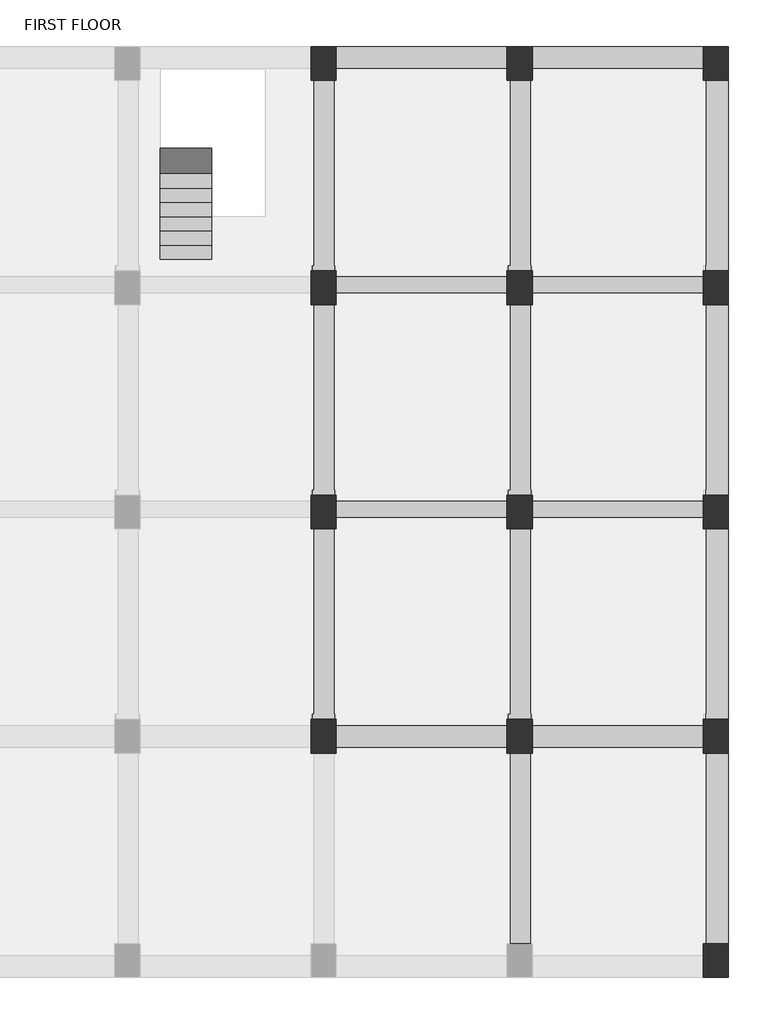
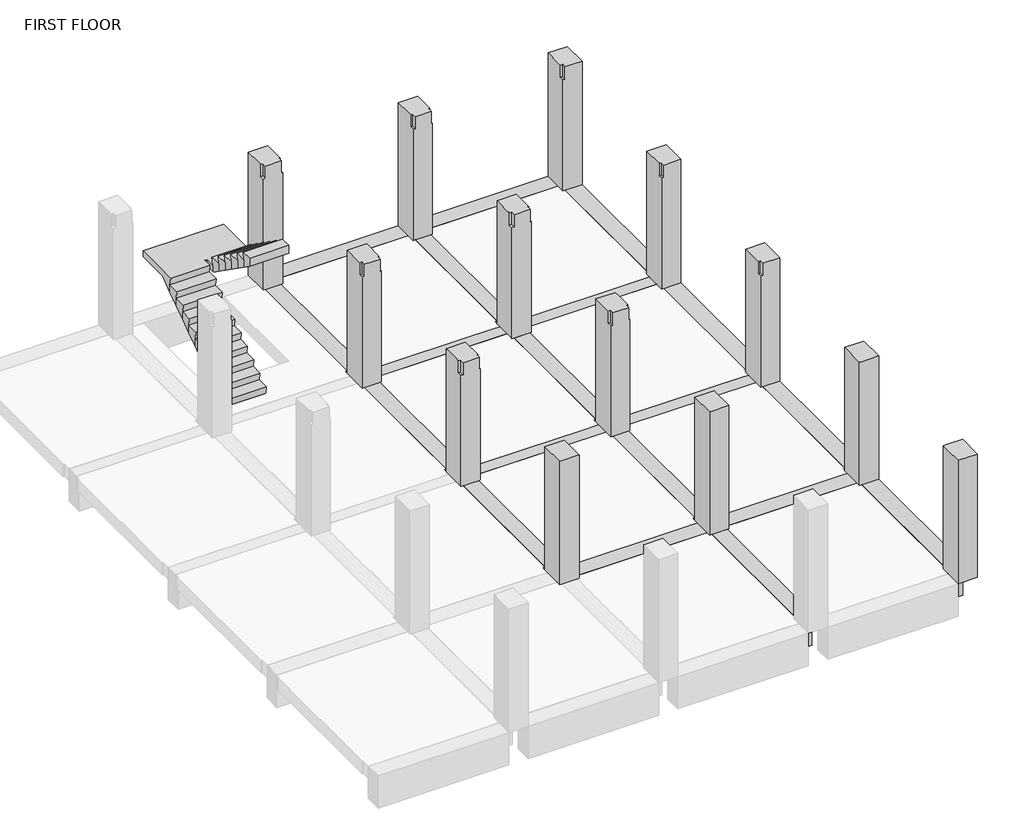
# One storey, part 4 of 4: 19 beams, 13 columns, 1 stair flight.
"""IFC4 building model written with IfcOpenShell, lengths in millimetres."""

from ifc_helpers import new_model, si_unit, origin, place, context, project, spatial, faceted_brep, element, save

model = new_model("IFC4")

# Units and contexts
model_context = context("Model", 3, world=origin())
ifc_project = project(units=[si_unit("LENGTHUNIT", "METRE", prefix="MILLI")], contexts=[model_context])

# Site, building, storey
site = spatial("IfcSite", under=ifc_project)
building = spatial("IfcBuilding", under=site)
storey = spatial("IfcBuildingStorey", under=building, Name="FIRST FLOOR", Elevation=3048.0)

# Beams
placement = place(None, origin())
element("IfcBeam", 1, ObjectType="M_Concrete-Rectangular Beam : 400 x 800mm", at=placement, inside=storey, context=model_context, shape_type="Brep", body=[
    faceted_brep([(7955.1115906, 15703.1212443, 3048.0), (8355.1115906, 15703.1212443, 3048.0), (8355.1115906, 19103.1212443, 3048.0), (7955.1115906, 19103.1212443, 3048.0), (7955.1115906, 15803.1212443, 3048.0), (7955.1115906, 15703.1212443, 2248.0), (7955.1115906, 19103.1212443, 2248.0), (8355.1115906, 15703.1212443, 2248.0), (8355.1115906, 19103.1212443, 2248.0)], [[[0, 1, 2, 3, 4]], [[5, 0, 4, 3, 6]], [[7, 5, 6, 8]], [[1, 7, 8, 2]], [[2, 8, 6, 3]], [[1, 0, 5, 7]]]),
])
element("IfcBeam", 2, ObjectType="M_Concrete-Rectangular Beam : 400 x 800mm", at=placement, inside=storey, context=model_context, shape_type="Brep", body=[
    faceted_brep([(7955.1115906, 11703.1212443, 3048.0), (8355.1115906, 11703.1212443, 3048.0), (8355.1115906, 15103.1212443, 3048.0), (7955.1115906, 15103.1212443, 3048.0), (7955.1115906, 11803.1212443, 3048.0), (7955.1115906, 11703.1212443, 2248.0), (7955.1115906, 15103.1212443, 2248.0), (8355.1115906, 11703.1212443, 2248.0), (8355.1115906, 15103.1212443, 2248.0)], [[[0, 1, 2, 3, 4]], [[5, 0, 4, 3, 6]], [[7, 5, 6, 8]], [[1, 7, 8, 2]], [[2, 8, 6, 3]], [[1, 0, 5, 7]]]),
])
element("IfcBeam", 3, ObjectType="M_Concrete-Rectangular Beam : 400 x 800mm", at=placement, inside=storey, context=model_context, shape_type="Brep", body=[
    faceted_brep([(7955.1115906, 7703.1212443, 3048.0), (8355.1115906, 7703.1212443, 3048.0), (8355.1115906, 11103.1212443, 3048.0), (7955.1115906, 11103.1212443, 3048.0), (7955.1115906, 7803.1212443, 3048.0), (7955.1115906, 7703.1212443, 2248.0), (7955.1115906, 11103.1212443, 2248.0), (8355.1115906, 7703.1212443, 2248.0), (8355.1115906, 11103.1212443, 2248.0)], [[[0, 1, 2, 3, 4]], [[5, 0, 4, 3, 6]], [[7, 5, 6, 8]], [[1, 7, 8, 2]], [[1, 0, 5, 7]], [[3, 2, 8, 6]]]),
])
element("IfcBeam", 4, ObjectType="M_Concrete-Rectangular Beam : 400 x 800mm", at=placement, inside=storey, context=model_context, shape_type="Brep", body=[
    faceted_brep([(8355.1115906, 7103.1212443, 3048.0), (7955.1115906, 7103.1212443, 3048.0), (7955.1115906, 3703.1212443, 3048.0), (8355.1115906, 3703.1212443, 3048.0), (7955.1115906, 7103.1212443, 2748.0), (7955.1115906, 7103.1212443, 2248.0), (7955.1115906, 3703.1212443, 2248.0), (7955.1115906, 3703.1212443, 2748.0), (8355.1115906, 7103.1212443, 2248.0), (8355.1115906, 3703.1212443, 2248.0)], [[[0, 1, 2, 3]], [[1, 4, 5, 6, 7, 2]], [[5, 8, 9, 6]], [[8, 0, 3, 9]], [[0, 8, 5, 4, 1]], [[3, 2, 7, 6, 9]]]),
])
element("IfcBeam", 5, ObjectType="M_Concrete-Rectangular Beam : 400 x 800mm", at=placement, inside=storey, context=model_context, shape_type="Brep", body=[
    faceted_brep([(1355.1115906, 19703.1212443, 3048.0), (1355.1115906, 19303.1212443, 3048.0), (4405.1115906, 19303.1212443, 3048.0), (4405.1115906, 19703.1212443, 3048.0), (1355.1115906, 19303.1212443, 2748.0), (1355.1115906, 19303.1212443, 2248.0), (4405.1115906, 19303.1212443, 2248.0), (4405.1115906, 19303.1212443, 2748.0), (1355.1115906, 19703.1212443, 2248.0), (4405.1115906, 19703.1212443, 2248.0)], [[[0, 1, 2, 3]], [[1, 4, 5, 6, 7, 2]], [[5, 8, 9, 6]], [[8, 0, 3, 9]], [[1, 0, 8, 5, 4]], [[3, 2, 7, 6, 9]]]),
])
element("IfcBeam", 6, ObjectType="M_Concrete-Rectangular Beam : 400 x 800mm", at=placement, inside=storey, context=model_context, shape_type="Brep", body=[
    faceted_brep([(4855.1115906, 19703.1212443, 3048.0), (4855.1115906, 19303.1212443, 3048.0), (7905.1115906, 19303.1212443, 3048.0), (7905.1115906, 19703.1212443, 3048.0), (4855.1115906, 19303.1212443, 2748.0), (4855.1115906, 19303.1212443, 2248.0), (7905.1115906, 19303.1212443, 2248.0), (7905.1115906, 19303.1212443, 2748.0), (4855.1115906, 19703.1212443, 2248.0), (7905.1115906, 19703.1212443, 2248.0)], [[[0, 1, 2, 3]], [[1, 4, 5, 6, 7, 2]], [[5, 8, 9, 6]], [[8, 0, 3, 9]], [[1, 0, 8, 5, 4]], [[3, 2, 7, 6, 9]]]),
])
element("IfcBeam", 7, ObjectType="M_Concrete-Rectangular Beam : 400 x 800mm", at=placement, inside=storey, context=model_context, shape_type="Brep", body=[
    faceted_brep([(1330.1115906, 15703.1212443, 3048.0), (1330.1115906, 15803.1212443, 3048.0), (1330.1115906, 19103.1212443, 3048.0), (955.1115906, 19103.1212443, 3048.0), (955.1115906, 15803.1212443, 3048.0), (930.1115906, 15803.1212443, 3048.0), (930.1115906, 15703.1212443, 3048.0), (930.1115906, 19103.1212443, 2248.0), (930.1115906, 15703.1212443, 2248.0), (930.1115906, 15803.1212443, 2748.0), (930.1115906, 19103.1212443, 2748.0), (1330.1115906, 19103.1212443, 2248.0), (1330.1115906, 15703.1212443, 2248.0), (955.1115906, 19103.1212443, 2748.0), (955.1115906, 15803.1212443, 2748.0)], [[[0, 1, 2, 3, 4, 5, 6]], [[7, 8, 6, 5, 9, 10]], [[7, 11, 12, 8]], [[11, 2, 1, 0, 12]], [[2, 11, 7, 10, 13, 3]], [[0, 6, 8, 12]], [[9, 14, 13, 10]], [[14, 4, 3, 13]], [[4, 14, 9, 5]]]),
])
element("IfcBeam", 8, ObjectType="M_Concrete-Rectangular Beam : 400 x 800mm", at=placement, inside=storey, context=model_context, shape_type="Brep", body=[
    faceted_brep([(1330.1115906, 11703.1212443, 3048.0), (1330.1115906, 11803.1212443, 3048.0), (1330.1115906, 15103.1212443, 3048.0), (955.1115906, 15103.1212443, 3048.0), (955.1115906, 11803.1212443, 3048.0), (930.1115906, 11803.1212443, 3048.0), (930.1115906, 11703.1212443, 3048.0), (930.1115906, 15103.1212443, 2248.0), (930.1115906, 11703.1212443, 2248.0), (930.1115906, 11803.1212443, 2748.0), (930.1115906, 15103.1212443, 2748.0), (1330.1115906, 15103.1212443, 2248.0), (1330.1115906, 11703.1212443, 2248.0), (955.1115906, 15103.1212443, 2748.0), (955.1115906, 11803.1212443, 2748.0)], [[[0, 1, 2, 3, 4, 5, 6]], [[7, 8, 6, 5, 9, 10]], [[8, 7, 11, 12]], [[2, 1, 0, 12, 11]], [[2, 11, 7, 10, 13, 3]], [[0, 6, 8, 12]], [[9, 14, 13, 10]], [[14, 4, 3, 13]], [[4, 14, 9, 5]]]),
])
element("IfcBeam", 9, ObjectType="M_Concrete-Rectangular Beam : 400 x 800mm", at=placement, inside=storey, context=model_context, shape_type="Brep", body=[
    faceted_brep([(1330.1115906, 7703.1212443, 3048.0), (1330.1115906, 7803.1212443, 3048.0), (1330.1115906, 11103.1212443, 3048.0), (955.1115906, 11103.1212443, 3048.0), (955.1115906, 7803.1212443, 3048.0), (930.1115906, 7803.1212443, 3048.0), (930.1115906, 7703.1212443, 3048.0), (930.1115906, 11103.1212443, 2248.0), (930.1115906, 7703.1212443, 2248.0), (930.1115906, 7803.1212443, 2748.0), (930.1115906, 11103.1212443, 2748.0), (1330.1115906, 11103.1212443, 2248.0), (1330.1115906, 7703.1212443, 2248.0), (955.1115906, 11103.1212443, 2748.0), (955.1115906, 7803.1212443, 2748.0)], [[[0, 1, 2, 3, 4, 5, 6]], [[7, 8, 6, 5, 9, 10]], [[7, 11, 12, 8]], [[11, 2, 1, 0, 12]], [[2, 11, 7, 10, 13, 3]], [[0, 6, 8, 12]], [[9, 14, 13, 10]], [[14, 4, 3, 13]], [[4, 14, 9, 5]]]),
])
element("IfcBeam", 10, ObjectType="M_Concrete-Rectangular Beam : 400 x 800mm", at=placement, inside=storey, context=model_context, shape_type="Brep", body=[
    faceted_brep([(4830.1115906, 15703.1212443, 3048.0), (4830.1115906, 15803.1212443, 3048.0), (4830.1115906, 19103.1212443, 3048.0), (4455.1115906, 19103.1212443, 3048.0), (4455.1115906, 15803.1212443, 3048.0), (4430.1115906, 15803.1212443, 3048.0), (4430.1115906, 15703.1212443, 3048.0), (4430.1115906, 19103.1212443, 2248.0), (4430.1115906, 15703.1212443, 2248.0), (4430.1115906, 15803.1212443, 2748.0), (4430.1115906, 19103.1212443, 2748.0), (4830.1115906, 19103.1212443, 2248.0), (4830.1115906, 15703.1212443, 2248.0), (4455.1115906, 19103.1212443, 2748.0), (4455.1115906, 15803.1212443, 2748.0)], [[[0, 1, 2, 3, 4, 5, 6]], [[7, 8, 6, 5, 9, 10]], [[8, 7, 11, 12]], [[2, 1, 0, 12, 11]], [[2, 11, 7, 10, 13, 3]], [[0, 6, 8, 12]], [[9, 14, 13, 10]], [[14, 4, 3, 13]], [[4, 14, 9, 5]]]),
])
element("IfcBeam", 11, ObjectType="M_Concrete-Rectangular Beam : 400 x 800mm", at=placement, inside=storey, context=model_context, shape_type="Brep", body=[
    faceted_brep([(4830.1115906, 11703.1212443, 3048.0), (4830.1115906, 11803.1212443, 3048.0), (4830.1115906, 15103.1212443, 3048.0), (4455.1115906, 15103.1212443, 3048.0), (4455.1115906, 11803.1212443, 3048.0), (4430.1115906, 11803.1212443, 3048.0), (4430.1115906, 11703.1212443, 3048.0), (4430.1115906, 15103.1212443, 2248.0), (4430.1115906, 11703.1212443, 2248.0), (4430.1115906, 11803.1212443, 2748.0), (4430.1115906, 15103.1212443, 2748.0), (4830.1115906, 15103.1212443, 2248.0), (4830.1115906, 11703.1212443, 2248.0), (4455.1115906, 15103.1212443, 2748.0), (4455.1115906, 11803.1212443, 2748.0)], [[[0, 1, 2, 3, 4, 5, 6]], [[7, 8, 6, 5, 9, 10]], [[7, 11, 12, 8]], [[11, 2, 1, 0, 12]], [[2, 11, 7, 10, 13, 3]], [[0, 6, 8, 12]], [[9, 14, 13, 10]], [[14, 4, 3, 13]], [[4, 14, 9, 5]]]),
])
element("IfcBeam", 12, ObjectType="M_Concrete-Rectangular Beam : 400 x 800mm", at=placement, inside=storey, context=model_context, shape_type="Brep", body=[
    faceted_brep([(4430.1115906, 7703.1212443, 3048.0), (4830.1115906, 7703.1212443, 3048.0), (4830.1115906, 7803.1212443, 3048.0), (4830.1115906, 11103.1212443, 3048.0), (4455.1115906, 11103.1212443, 3048.0), (4455.1115906, 7803.1212443, 3048.0), (4430.1115906, 7803.1212443, 3048.0), (4430.1115906, 7703.1212443, 2248.0), (4430.1115906, 7803.1212443, 2748.0), (4430.1115906, 11103.1212443, 2748.0), (4430.1115906, 11103.1212443, 2248.0), (4830.1115906, 7703.1212443, 2248.0), (4830.1115906, 11103.1212443, 2248.0), (4455.1115906, 11103.1212443, 2748.0), (4455.1115906, 7803.1212443, 2748.0)], [[[0, 1, 2, 3, 4, 5, 6]], [[7, 0, 6, 8, 9, 10]], [[11, 7, 10, 12]], [[1, 11, 12, 3, 2]], [[1, 0, 7, 11]], [[12, 10, 9, 13, 4, 3]], [[8, 14, 13, 9]], [[14, 5, 4, 13]], [[5, 14, 8, 6]]]),
])
element("IfcBeam", 13, ObjectType="M_Concrete-Rectangular Beam : 400 x 800mm", at=placement, inside=storey, context=model_context, shape_type="Brep", body=[
    faceted_brep([(4830.1115906, 3703.1212443, 3048.0), (4830.1115906, 7103.1212443, 3048.0), (4455.1115906, 7103.1212443, 3048.0), (4455.1115906, 3703.1212443, 3048.0), (4430.1115906, 7103.1212443, 2248.0), (4430.1115906, 3703.1212443, 2248.0), (4430.1115906, 3703.1212443, 2748.0), (4430.1115906, 7103.1212443, 2748.0), (4830.1115906, 7103.1212443, 2248.0), (4830.1115906, 3703.1212443, 2248.0), (4830.1115906, 7103.1212443, 2748.0), (4830.1115906, 3703.1212443, 2748.0), (4455.1115906, 7103.1212443, 2748.0), (4455.1115906, 3703.1212443, 2748.0)], [[[0, 1, 2, 3]], [[4, 5, 6, 7]], [[4, 8, 9, 5]], [[8, 10, 1, 0, 11, 9]], [[1, 10, 8, 4, 7, 12, 2]], [[5, 9, 11, 0, 3, 13, 6]], [[13, 12, 7, 6]], [[12, 13, 3, 2]]]),
])
element("IfcBeam", 14, ObjectType="M_Concrete-Rectangular Beam : 400 x 800mm", at=placement, inside=storey, context=model_context, shape_type="Brep", body=[
    faceted_brep([(4405.1115906, 15603.1212443, 3048.0), (1355.1115906, 15603.1212443, 3048.0), (1355.1115906, 15303.1212443, 3048.0), (4405.1115906, 15303.1212443, 3048.0), (1355.1115906, 15203.1212443, 2248.0), (4405.1115906, 15203.1212443, 2248.0), (4405.1115906, 15203.1212443, 2748.0), (1355.1115906, 15203.1212443, 2748.0), (1355.1115906, 15603.1212443, 2248.0), (4405.1115906, 15603.1212443, 2248.0), (1355.1115906, 15603.1212443, 2748.0), (4405.1115906, 15603.1212443, 2748.0), (1355.1115906, 15303.1212443, 2748.0), (4405.1115906, 15303.1212443, 2748.0)], [[[0, 1, 2, 3]], [[4, 5, 6, 7]], [[4, 8, 9, 5]], [[8, 10, 1, 0, 11, 9]], [[8, 4, 7, 12, 2, 1, 10]], [[5, 9, 11, 0, 3, 13, 6]], [[13, 12, 7, 6]], [[12, 13, 3, 2]]]),
])
element("IfcBeam", 15, ObjectType="M_Concrete-Rectangular Beam : 400 x 800mm", at=placement, inside=storey, context=model_context, shape_type="Brep", body=[
    faceted_brep([(7905.1115906, 15603.1212443, 3048.0), (4855.1115906, 15603.1212443, 3048.0), (4855.1115906, 15303.1212443, 3048.0), (7905.1115906, 15303.1212443, 3048.0), (4855.1115906, 15203.1212443, 2248.0), (7905.1115906, 15203.1212443, 2248.0), (7905.1115906, 15203.1212443, 2748.0), (4855.1115906, 15203.1212443, 2748.0), (4855.1115906, 15603.1212443, 2248.0), (7905.1115906, 15603.1212443, 2248.0), (4855.1115906, 15603.1212443, 2748.0), (7905.1115906, 15603.1212443, 2748.0), (4855.1115906, 15303.1212443, 2748.0), (7905.1115906, 15303.1212443, 2748.0)], [[[0, 1, 2, 3]], [[4, 5, 6, 7]], [[4, 8, 9, 5]], [[8, 10, 1, 0, 11, 9]], [[8, 4, 7, 12, 2, 1, 10]], [[5, 9, 11, 0, 3, 13, 6]], [[13, 12, 7, 6]], [[12, 13, 3, 2]]]),
])
element("IfcBeam", 16, ObjectType="M_Concrete-Rectangular Beam : 400 x 800mm", at=placement, inside=storey, context=model_context, shape_type="Brep", body=[
    faceted_brep([(7905.1115906, 11603.1212443, 3048.0), (4855.1115906, 11603.1212443, 3048.0), (4855.1115906, 11303.1212443, 3048.0), (7905.1115906, 11303.1212443, 3048.0), (4855.1115906, 11603.1212443, 2248.0), (4855.1115906, 11603.1212443, 2748.0), (7905.1115906, 11603.1212443, 2748.0), (7905.1115906, 11603.1212443, 2248.0), (4855.1115906, 11203.1212443, 2248.0), (7905.1115906, 11203.1212443, 2248.0), (7905.1115906, 11203.1212443, 2748.0), (4855.1115906, 11203.1212443, 2748.0), (4855.1115906, 11303.1212443, 2748.0), (7905.1115906, 11303.1212443, 2748.0)], [[[0, 1, 2, 3]], [[4, 5, 1, 0, 6, 7]], [[8, 4, 7, 9]], [[8, 9, 10, 11]], [[1, 5, 4, 8, 11, 12, 2]], [[7, 6, 0, 3, 13, 10, 9]], [[13, 12, 11, 10]], [[12, 13, 3, 2]]]),
])
element("IfcBeam", 17, ObjectType="M_Concrete-Rectangular Beam : 400 x 800mm", at=placement, inside=storey, context=model_context, shape_type="Brep", body=[
    faceted_brep([(4405.1115906, 11603.1212443, 3048.0), (1355.1115906, 11603.1212443, 3048.0), (1355.1115906, 11303.1212443, 3048.0), (4405.1115906, 11303.1212443, 3048.0), (1355.1115906, 11603.1212443, 2248.0), (1355.1115906, 11603.1212443, 2748.0), (4405.1115906, 11603.1212443, 2748.0), (4405.1115906, 11603.1212443, 2248.0), (1355.1115906, 11203.1212443, 2248.0), (4405.1115906, 11203.1212443, 2248.0), (4405.1115906, 11203.1212443, 2748.0), (1355.1115906, 11203.1212443, 2748.0), (1355.1115906, 11303.1212443, 2748.0), (4405.1115906, 11303.1212443, 2748.0)], [[[0, 1, 2, 3]], [[4, 5, 1, 0, 6, 7]], [[8, 4, 7, 9]], [[8, 9, 10, 11]], [[1, 5, 4, 8, 11, 12, 2]], [[7, 6, 0, 3, 13, 10, 9]], [[13, 12, 11, 10]], [[12, 13, 3, 2]]]),
])
element("IfcBeam", 18, ObjectType="M_Concrete-Rectangular Beam : 400 x 800mm", at=placement, inside=storey, context=model_context, shape_type="Brep", body=[
    faceted_brep([(1355.1115906, 7603.1212443, 3048.0), (1355.1115906, 7203.1212443, 3048.0), (4405.1115906, 7203.1212443, 3048.0), (4405.1115906, 7603.1212443, 3048.0), (1355.1115906, 7203.1212443, 2748.0), (1355.1115906, 7203.1212443, 2248.0), (4405.1115906, 7203.1212443, 2248.0), (4405.1115906, 7203.1212443, 2748.0), (1355.1115906, 7603.1212443, 2248.0), (4405.1115906, 7603.1212443, 2248.0), (1355.1115906, 7603.1212443, 2748.0), (4405.1115906, 7603.1212443, 2748.0)], [[[0, 1, 2, 3]], [[1, 4, 5, 6, 7, 2]], [[5, 8, 9, 6]], [[8, 10, 0, 3, 11, 9]], [[1, 0, 10, 8, 5, 4]], [[3, 2, 7, 6, 9, 11]]]),
])
element("IfcBeam", 19, ObjectType="M_Concrete-Rectangular Beam : 400 x 800mm", at=placement, inside=storey, context=model_context, shape_type="Brep", body=[
    faceted_brep([(4855.1115906, 7603.1212443, 3048.0), (4855.1115906, 7203.1212443, 3048.0), (7905.1115906, 7203.1212443, 3048.0), (7905.1115906, 7603.1212443, 3048.0), (4855.1115906, 7203.1212443, 2748.0), (4855.1115906, 7203.1212443, 2248.0), (7905.1115906, 7203.1212443, 2248.0), (7905.1115906, 7203.1212443, 2748.0), (4855.1115906, 7603.1212443, 2248.0), (7905.1115906, 7603.1212443, 2248.0), (4855.1115906, 7603.1212443, 2748.0), (7905.1115906, 7603.1212443, 2748.0)], [[[0, 1, 2, 3]], [[1, 4, 5, 6, 7, 2]], [[5, 8, 9, 6]], [[8, 10, 0, 3, 11, 9]], [[1, 0, 10, 8, 5, 4]], [[3, 2, 7, 6, 9, 11]]]),
])

# Columns
element("IfcColumn", 20, ObjectType="M_Concrete-Rectangular-Column : 450 x 600mm", at=placement, inside=storey, context=model_context, shape_type="Brep", body=[
    faceted_brep([(1355.1115906, 19703.1212443, 3048.0), (1355.1115906, 19103.1212443, 3048.0), (905.1115906, 19103.1212443, 3048.0), (905.1115906, 19703.1212443, 3048.0), (1355.1115906, 19703.1212443, 6096.0), (1355.1115906, 19303.1212443, 6096.0), (1355.1115906, 19203.1212443, 6096.0), (1355.1115906, 19203.1212443, 5796.0), (1355.1115906, 19103.1212443, 5796.0), (1330.1115906, 19103.1212443, 5796.0), (1330.1115906, 19103.1212443, 6096.0), (955.1115906, 19103.1212443, 6096.0), (955.1115906, 19103.1212443, 5796.0), (905.1115906, 19103.1212443, 5796.0), (905.1115906, 19203.1212443, 5796.0), (905.1115906, 19203.1212443, 6096.0), (905.1115906, 19303.1212443, 6096.0), (905.1115906, 19703.1212443, 6096.0), (955.1115906, 19203.1212443, 6096.0), (1330.1115906, 19203.1212443, 6096.0), (1330.1115906, 19203.1212443, 5796.0), (955.1115906, 19203.1212443, 5796.0)], [[[0, 1, 2, 3]], [[1, 0, 4, 5, 6, 7, 8]], [[2, 1, 8, 9, 10, 11, 12, 13]], [[3, 2, 13, 14, 15, 16, 17]], [[0, 3, 17, 4]], [[4, 17, 16, 15, 18, 11, 10, 19, 6, 5]], [[7, 20, 9, 8]], [[20, 19, 10, 9]], [[20, 7, 6, 19]], [[21, 14, 13, 12]], [[18, 21, 12, 11]], [[14, 21, 18, 15]]]),
])
element("IfcColumn", 21, ObjectType="M_Concrete-Rectangular-Column : 450 x 600mm", at=placement, inside=storey, context=model_context, shape_type="Brep", body=[
    faceted_brep([(4855.1115906, 19703.1212443, 3048.0), (4855.1115906, 19103.1212443, 3048.0), (4405.1115906, 19103.1212443, 3048.0), (4405.1115906, 19703.1212443, 3048.0), (4855.1115906, 19703.1212443, 6096.0), (4855.1115906, 19303.1212443, 6096.0), (4855.1115906, 19203.1212443, 6096.0), (4855.1115906, 19203.1212443, 5796.0), (4855.1115906, 19103.1212443, 5796.0), (4830.1115906, 19103.1212443, 5796.0), (4830.1115906, 19103.1212443, 6096.0), (4455.1115906, 19103.1212443, 6096.0), (4455.1115906, 19103.1212443, 5796.0), (4405.1115906, 19103.1212443, 5796.0), (4405.1115906, 19203.1212443, 5796.0), (4405.1115906, 19203.1212443, 6096.0), (4405.1115906, 19303.1212443, 6096.0), (4405.1115906, 19703.1212443, 6096.0), (4455.1115906, 19203.1212443, 6096.0), (4830.1115906, 19203.1212443, 6096.0), (4830.1115906, 19203.1212443, 5796.0), (4455.1115906, 19203.1212443, 5796.0)], [[[0, 1, 2, 3]], [[1, 0, 4, 5, 6, 7, 8]], [[2, 1, 8, 9, 10, 11, 12, 13]], [[3, 2, 13, 14, 15, 16, 17]], [[0, 3, 17, 4]], [[4, 17, 16, 15, 18, 11, 10, 19, 6, 5]], [[7, 20, 9, 8]], [[20, 19, 10, 9]], [[20, 7, 6, 19]], [[21, 14, 13, 12]], [[18, 21, 12, 11]], [[14, 21, 18, 15]]]),
])
element("IfcColumn", 22, ObjectType="M_Concrete-Rectangular-Column : 450 x 600mm", at=placement, inside=storey, context=model_context, shape_type="Brep", body=[
    faceted_brep([(8355.1115906, 19703.1212443, 3048.0), (8355.1115906, 19103.1212443, 3048.0), (7905.1115906, 19103.1212443, 3048.0), (7905.1115906, 19703.1212443, 3048.0), (8355.1115906, 19703.1212443, 6096.0), (8355.1115906, 19103.1212443, 6096.0), (7955.1115906, 19103.1212443, 6096.0), (7955.1115906, 19103.1212443, 5796.0), (7905.1115906, 19103.1212443, 5796.0), (7905.1115906, 19203.1212443, 5796.0), (7905.1115906, 19203.1212443, 6096.0), (7905.1115906, 19303.1212443, 6096.0), (7905.1115906, 19703.1212443, 6096.0), (7955.1115906, 19203.1212443, 6096.0), (7955.1115906, 19203.1212443, 5796.0)], [[[0, 1, 2, 3]], [[1, 0, 4, 5]], [[2, 1, 5, 6, 7, 8]], [[3, 2, 8, 9, 10, 11, 12]], [[0, 3, 12, 4]], [[5, 4, 12, 11, 10, 13, 6]], [[14, 9, 8, 7]], [[13, 14, 7, 6]], [[9, 14, 13, 10]]]),
])
element("IfcColumn", 23, ObjectType="M_Concrete-Rectangular-Column : 450 x 600mm", at=placement, inside=storey, context=model_context, shape_type="Brep", body=[
    faceted_brep([(1355.1115906, 15703.1212443, 3048.0), (1355.1115906, 15103.1212443, 3048.0), (905.1115906, 15103.1212443, 3048.0), (905.1115906, 15703.1212443, 3048.0), (1355.1115906, 15703.1212443, 5796.0), (1355.1115906, 15703.1212443, 6096.0), (1355.1115906, 15603.1212443, 6096.0), (1355.1115906, 15303.1212443, 6096.0), (1355.1115906, 15203.1212443, 6096.0), (1355.1115906, 15203.1212443, 5796.0), (1355.1115906, 15103.1212443, 5796.0), (1330.1115906, 15103.1212443, 5796.0), (1330.1115906, 15103.1212443, 6096.0), (955.1115906, 15103.1212443, 6096.0), (955.1115906, 15103.1212443, 5796.0), (905.1115906, 15103.1212443, 5796.0), (905.1115906, 15203.1212443, 5796.0), (905.1115906, 15203.1212443, 6096.0), (905.1115906, 15303.1212443, 6096.0), (905.1115906, 15603.1212443, 6096.0), (905.1115906, 15703.1212443, 6096.0), (905.1115906, 15703.1212443, 5796.0), (955.1115906, 15203.1212443, 6096.0), (1330.1115906, 15203.1212443, 6096.0), (1330.1115906, 15203.1212443, 5796.0), (955.1115906, 15203.1212443, 5796.0)], [[[0, 1, 2, 3]], [[1, 0, 4, 5, 6, 7, 8, 9, 10]], [[2, 1, 10, 11, 12, 13, 14, 15]], [[3, 2, 15, 16, 17, 18, 19, 20, 21]], [[0, 3, 21, 20, 5, 4]], [[5, 20, 19, 18, 17, 22, 13, 12, 23, 8, 7, 6]], [[9, 24, 11, 10]], [[24, 23, 12, 11]], [[24, 9, 8, 23]], [[25, 16, 15, 14]], [[22, 25, 14, 13]], [[16, 25, 22, 17]]]),
])
element("IfcColumn", 24, ObjectType="M_Concrete-Rectangular-Column : 450 x 600mm", at=placement, inside=storey, context=model_context, shape_type="Brep", body=[
    faceted_brep([(4855.1115906, 15703.1212443, 3048.0), (4855.1115906, 15103.1212443, 3048.0), (4405.1115906, 15103.1212443, 3048.0), (4405.1115906, 15703.1212443, 3048.0), (4855.1115906, 15703.1212443, 5796.0), (4855.1115906, 15703.1212443, 6096.0), (4855.1115906, 15603.1212443, 6096.0), (4855.1115906, 15303.1212443, 6096.0), (4855.1115906, 15203.1212443, 6096.0), (4855.1115906, 15203.1212443, 5796.0), (4855.1115906, 15103.1212443, 5796.0), (4830.1115906, 15103.1212443, 5796.0), (4830.1115906, 15103.1212443, 6096.0), (4455.1115906, 15103.1212443, 6096.0), (4455.1115906, 15103.1212443, 5796.0), (4405.1115906, 15103.1212443, 5796.0), (4405.1115906, 15203.1212443, 5796.0), (4405.1115906, 15203.1212443, 6096.0), (4405.1115906, 15303.1212443, 6096.0), (4405.1115906, 15603.1212443, 6096.0), (4405.1115906, 15703.1212443, 6096.0), (4405.1115906, 15703.1212443, 5796.0), (4455.1115906, 15203.1212443, 6096.0), (4830.1115906, 15203.1212443, 6096.0), (4830.1115906, 15203.1212443, 5796.0), (4455.1115906, 15203.1212443, 5796.0)], [[[0, 1, 2, 3]], [[1, 0, 4, 5, 6, 7, 8, 9, 10]], [[2, 1, 10, 11, 12, 13, 14, 15]], [[3, 2, 15, 16, 17, 18, 19, 20, 21]], [[0, 3, 21, 20, 5, 4]], [[5, 20, 19, 18, 17, 22, 13, 12, 23, 8, 7, 6]], [[9, 24, 11, 10]], [[24, 23, 12, 11]], [[24, 9, 8, 23]], [[25, 16, 15, 14]], [[22, 25, 14, 13]], [[16, 25, 22, 17]]]),
])
element("IfcColumn", 25, ObjectType="M_Concrete-Rectangular-Column : 450 x 600mm", at=placement, inside=storey, context=model_context, shape_type="Brep", body=[
    faceted_brep([(8355.1115906, 15703.1212443, 3048.0), (8355.1115906, 15103.1212443, 3048.0), (7905.1115906, 15103.1212443, 3048.0), (7905.1115906, 15703.1212443, 3048.0), (8355.1115906, 15703.1212443, 6096.0), (8355.1115906, 15103.1212443, 6096.0), (7955.1115906, 15103.1212443, 6096.0), (7955.1115906, 15103.1212443, 5796.0), (7905.1115906, 15103.1212443, 5796.0), (7905.1115906, 15203.1212443, 5796.0), (7905.1115906, 15203.1212443, 6096.0), (7905.1115906, 15303.1212443, 6096.0), (7905.1115906, 15603.1212443, 6096.0), (7905.1115906, 15703.1212443, 6096.0), (7905.1115906, 15703.1212443, 5796.0), (7955.1115906, 15203.1212443, 6096.0), (7955.1115906, 15203.1212443, 5796.0)], [[[0, 1, 2, 3]], [[1, 0, 4, 5]], [[2, 1, 5, 6, 7, 8]], [[3, 2, 8, 9, 10, 11, 12, 13, 14]], [[0, 3, 14, 13, 4]], [[5, 4, 13, 12, 11, 10, 15, 6]], [[16, 9, 8, 7]], [[15, 16, 7, 6]], [[9, 16, 15, 10]]]),
])
element("IfcColumn", 26, ObjectType="M_Concrete-Rectangular-Column : 450 x 600mm", at=placement, inside=storey, context=model_context, shape_type="Brep", body=[
    faceted_brep([(1355.1115906, 11703.1212443, 3048.0), (1355.1115906, 11103.1212443, 3048.0), (905.1115906, 11103.1212443, 3048.0), (905.1115906, 11703.1212443, 3048.0), (1355.1115906, 11703.1212443, 5796.0), (1355.1115906, 11703.1212443, 6096.0), (1355.1115906, 11603.1212443, 6096.0), (1355.1115906, 11303.1212443, 6096.0), (1355.1115906, 11203.1212443, 6096.0), (1355.1115906, 11203.1212443, 5796.0), (1355.1115906, 11103.1212443, 5796.0), (1330.1115906, 11103.1212443, 5796.0), (1330.1115906, 11103.1212443, 6096.0), (955.1115906, 11103.1212443, 6096.0), (955.1115906, 11103.1212443, 5796.0), (905.1115906, 11103.1212443, 5796.0), (905.1115906, 11203.1212443, 5796.0), (905.1115906, 11203.1212443, 6096.0), (905.1115906, 11303.1212443, 6096.0), (905.1115906, 11603.1212443, 6096.0), (905.1115906, 11703.1212443, 6096.0), (905.1115906, 11703.1212443, 5796.0), (955.1115906, 11203.1212443, 6096.0), (1330.1115906, 11203.1212443, 6096.0), (1330.1115906, 11203.1212443, 5796.0), (955.1115906, 11203.1212443, 5796.0)], [[[0, 1, 2, 3]], [[1, 0, 4, 5, 6, 7, 8, 9, 10]], [[2, 1, 10, 11, 12, 13, 14, 15]], [[3, 2, 15, 16, 17, 18, 19, 20, 21]], [[0, 3, 21, 20, 5, 4]], [[5, 20, 19, 18, 17, 22, 13, 12, 23, 8, 7, 6]], [[9, 24, 11, 10]], [[24, 23, 12, 11]], [[24, 9, 8, 23]], [[25, 16, 15, 14]], [[22, 25, 14, 13]], [[16, 25, 22, 17]]]),
])
element("IfcColumn", 27, ObjectType="M_Concrete-Rectangular-Column : 450 x 600mm", at=placement, inside=storey, context=model_context, shape_type="Brep", body=[
    faceted_brep([(4855.1115906, 11703.1212443, 3048.0), (4855.1115906, 11103.1212443, 3048.0), (4405.1115906, 11103.1212443, 3048.0), (4405.1115906, 11703.1212443, 3048.0), (4855.1115906, 11703.1212443, 5796.0), (4855.1115906, 11703.1212443, 6096.0), (4855.1115906, 11603.1212443, 6096.0), (4855.1115906, 11303.1212443, 6096.0), (4855.1115906, 11203.1212443, 6096.0), (4855.1115906, 11203.1212443, 5796.0), (4855.1115906, 11103.1212443, 5796.0), (4830.1115906, 11103.1212443, 5796.0), (4830.1115906, 11103.1212443, 6096.0), (4455.1115906, 11103.1212443, 6096.0), (4455.1115906, 11103.1212443, 5796.0), (4405.1115906, 11103.1212443, 5796.0), (4405.1115906, 11203.1212443, 5796.0), (4405.1115906, 11203.1212443, 6096.0), (4405.1115906, 11303.1212443, 6096.0), (4405.1115906, 11603.1212443, 6096.0), (4405.1115906, 11703.1212443, 6096.0), (4405.1115906, 11703.1212443, 5796.0), (4455.1115906, 11203.1212443, 6096.0), (4830.1115906, 11203.1212443, 6096.0), (4830.1115906, 11203.1212443, 5796.0), (4455.1115906, 11203.1212443, 5796.0)], [[[0, 1, 2, 3]], [[1, 0, 4, 5, 6, 7, 8, 9, 10]], [[2, 1, 10, 11, 12, 13, 14, 15]], [[3, 2, 15, 16, 17, 18, 19, 20, 21]], [[0, 3, 21, 20, 5, 4]], [[5, 20, 19, 18, 17, 22, 13, 12, 23, 8, 7, 6]], [[9, 24, 11, 10]], [[24, 23, 12, 11]], [[24, 9, 8, 23]], [[25, 16, 15, 14]], [[22, 25, 14, 13]], [[16, 25, 22, 17]]]),
])
element("IfcColumn", 28, ObjectType="M_Concrete-Rectangular-Column : 450 x 600mm", at=placement, inside=storey, context=model_context, shape_type="Brep", body=[
    faceted_brep([(8355.1115906, 11703.1212443, 3048.0), (8355.1115906, 11103.1212443, 3048.0), (7905.1115906, 11103.1212443, 3048.0), (7905.1115906, 11703.1212443, 3048.0), (8355.1115906, 11703.1212443, 6096.0), (8355.1115906, 11103.1212443, 6096.0), (7955.1115906, 11103.1212443, 6096.0), (7955.1115906, 11103.1212443, 5796.0), (7905.1115906, 11103.1212443, 5796.0), (7905.1115906, 11203.1212443, 5796.0), (7905.1115906, 11203.1212443, 6096.0), (7905.1115906, 11303.1212443, 6096.0), (7905.1115906, 11603.1212443, 6096.0), (7905.1115906, 11703.1212443, 6096.0), (7905.1115906, 11703.1212443, 5796.0), (7955.1115906, 11203.1212443, 6096.0), (7955.1115906, 11203.1212443, 5796.0)], [[[0, 1, 2, 3]], [[1, 0, 4, 5]], [[2, 1, 5, 6, 7, 8]], [[3, 2, 8, 9, 10, 11, 12, 13, 14]], [[0, 3, 14, 13, 4]], [[5, 4, 13, 12, 11, 10, 15, 6]], [[16, 9, 8, 7]], [[15, 16, 7, 6]], [[9, 16, 15, 10]]]),
])
element("IfcColumn", 29, ObjectType="M_Concrete-Rectangular-Column : 450 x 600mm", at=placement, inside=storey, context=model_context, shape_type="Brep", body=[
    faceted_brep([(1355.1115906, 7703.1212443, 3048.0), (1355.1115906, 7103.1212443, 3048.0), (905.1115906, 7103.1212443, 3048.0), (905.1115906, 7703.1212443, 3048.0), (1355.1115906, 7703.1212443, 5796.0), (1355.1115906, 7703.1212443, 6096.0), (1355.1115906, 7603.1212443, 6096.0), (1355.1115906, 7203.1212443, 6096.0), (1355.1115906, 7103.1212443, 6096.0), (1355.1115906, 7103.1212443, 5796.0), (1330.1115906, 7103.1212443, 6096.0), (955.1115906, 7103.1212443, 6096.0), (905.1115906, 7103.1212443, 6096.0), (905.1115906, 7103.1212443, 5796.0), (905.1115906, 7203.1212443, 6096.0), (905.1115906, 7603.1212443, 6096.0), (905.1115906, 7703.1212443, 6096.0), (905.1115906, 7703.1212443, 5796.0)], [[[0, 1, 2, 3]], [[1, 0, 4, 5, 6, 7, 8, 9]], [[2, 1, 9, 8, 10, 11, 12, 13]], [[3, 2, 13, 12, 14, 15, 16, 17]], [[0, 3, 17, 16, 5, 4]], [[5, 16, 15, 14, 12, 11, 10, 8, 7, 6]]]),
])
element("IfcColumn", 30, ObjectType="M_Concrete-Rectangular-Column : 450 x 600mm", at=placement, inside=storey, context=model_context, shape_type="Brep", body=[
    faceted_brep([(4855.1115906, 7703.1212443, 3048.0), (4855.1115906, 7103.1212443, 3048.0), (4405.1115906, 7103.1212443, 3048.0), (4405.1115906, 7703.1212443, 3048.0), (4855.1115906, 7703.1212443, 5796.0), (4855.1115906, 7703.1212443, 6096.0), (4855.1115906, 7603.1212443, 6096.0), (4855.1115906, 7203.1212443, 6096.0), (4855.1115906, 7103.1212443, 6096.0), (4855.1115906, 7103.1212443, 5796.0), (4830.1115906, 7103.1212443, 6096.0), (4455.1115906, 7103.1212443, 6096.0), (4405.1115906, 7103.1212443, 6096.0), (4405.1115906, 7103.1212443, 5796.0), (4405.1115906, 7203.1212443, 6096.0), (4405.1115906, 7603.1212443, 6096.0), (4405.1115906, 7703.1212443, 6096.0), (4405.1115906, 7703.1212443, 5796.0)], [[[0, 1, 2, 3]], [[1, 0, 4, 5, 6, 7, 8, 9]], [[2, 1, 9, 8, 10, 11, 12, 13]], [[3, 2, 13, 12, 14, 15, 16, 17]], [[0, 3, 17, 16, 5, 4]], [[5, 16, 15, 14, 12, 11, 10, 8, 7, 6]]]),
])
element("IfcColumn", 31, ObjectType="M_Concrete-Rectangular-Column : 450 x 600mm", at=placement, inside=storey, context=model_context, shape_type="Brep", body=[
    faceted_brep([(8355.1115906, 7703.1212443, 3048.0), (8355.1115906, 7103.1212443, 3048.0), (7905.1115906, 7103.1212443, 3048.0), (7905.1115906, 7703.1212443, 3048.0), (8355.1115906, 7703.1212443, 6096.0), (8355.1115906, 7103.1212443, 6096.0), (7955.1115906, 7103.1212443, 6096.0), (7905.1115906, 7103.1212443, 6096.0), (7905.1115906, 7103.1212443, 5796.0), (7905.1115906, 7203.1212443, 6096.0), (7905.1115906, 7603.1212443, 6096.0), (7905.1115906, 7703.1212443, 6096.0), (7905.1115906, 7703.1212443, 5796.0)], [[[0, 1, 2, 3]], [[1, 0, 4, 5]], [[2, 1, 5, 6, 7, 8]], [[3, 2, 8, 7, 9, 10, 11, 12]], [[0, 3, 12, 11, 4]], [[5, 4, 11, 10, 9, 7, 6]]]),
])
element("IfcColumn", 32, ObjectType="M_Concrete-Rectangular-Column : 450 x 600mm", at=placement, inside=storey, context=model_context, shape_type="Brep", body=[
    faceted_brep([(8355.1115906, 3703.1212443, 3048.0), (8355.1115906, 3103.1212443, 3048.0), (7905.1115906, 3103.1212443, 3048.0), (7905.1115906, 3703.1212443, 3048.0), (8355.1115906, 3703.1212443, 6096.0), (8355.1115906, 3103.1212443, 6096.0), (7905.1115906, 3103.1212443, 6096.0), (7905.1115906, 3503.1212443, 6096.0), (7905.1115906, 3703.1212443, 6096.0), (7905.1115906, 3703.1212443, 5796.0), (7955.1115906, 3703.1212443, 6096.0)], [[[0, 1, 2, 3]], [[1, 0, 4, 5]], [[2, 1, 5, 6]], [[3, 2, 6, 7, 8, 9]], [[0, 3, 9, 8, 10, 4]], [[5, 4, 10, 8, 7, 6]]]),
])

# Stair flight
element("IfcStairFlight", 33, ObjectType="25 mm Nosing", at=placement, inside=storey, context=model_context, shape_type="Brep", body=[
    faceted_brep([(-1784.8884094, 15908.7212443, 3227.2941176), (-870.4884094, 15908.7212443, 3227.2941176), (-870.4884094, 16187.7212443, 3227.2941176), (-1784.8884094, 16187.7212443, 3227.2941176), (-1784.8884094, 16187.7212443, 3048.0), (-1784.8884094, 15933.7212443, 3048.0), (-870.4884094, 15933.7212443, 3048.0), (-870.4884094, 16187.7212443, 3048.0), (-1784.8884094, 16162.7212443, 3406.5882353), (-870.4884094, 16162.7212443, 3406.5882353), (-870.4884094, 16441.7212443, 3406.5882353), (-1784.8884094, 16441.7212443, 3406.5882353), (-1784.8884094, 16441.7212443, 3222.9824819), (-1784.8884094, 16193.8293949, 3048.0), (-870.4884094, 16193.8293949, 3048.0), (-870.4884094, 16441.7212443, 3222.9824819), (-1784.8884094, 16416.7212443, 3585.8823529), (-870.4884094, 16416.7212443, 3585.8823529), (-870.4884094, 16695.7212443, 3585.8823529), (-1784.8884094, 16695.7212443, 3585.8823529), (-1784.8884094, 16695.7212443, 3402.2765996), (-870.4884094, 16695.7212443, 3402.2765996), (-1784.8884094, 16670.7212443, 3765.1764706), (-870.4884094, 16670.7212443, 3765.1764706), (-870.4884094, 16949.7212443, 3765.1764706), (-1784.8884094, 16949.7212443, 3765.1764706), (-1784.8884094, 16949.7212443, 3581.5707172), (-870.4884094, 16949.7212443, 3581.5707172), (-1784.8884094, 16924.7212443, 3944.4705882), (-870.4884094, 16924.7212443, 3944.4705882), (-870.4884094, 17203.7212443, 3944.4705882), (-1784.8884094, 17203.7212443, 3944.4705882), (-1784.8884094, 17203.7212443, 3760.8648349), (-870.4884094, 17203.7212443, 3760.8648349), (-1784.8884094, 17178.7212443, 4123.7647059), (-870.4884094, 17178.7212443, 4123.7647059), (-870.4884094, 17457.7212443, 4123.7647059), (-1784.8884094, 17457.7212443, 4123.7647059), (-1784.8884094, 17457.7212443, 3940.1589525), (-870.4884094, 17457.7212443, 3940.1589525), (-1784.8884094, 17432.7212443, 4303.0588235), (-870.4884094, 17432.7212443, 4303.0588235), (-870.4884094, 17711.7212443, 4303.0588235), (-1784.8884094, 17711.7212443, 4303.0588235), (-1784.8884094, 17711.7212443, 4119.4530702), (-870.4884094, 17711.7212443, 4119.4530702), (-1784.8884094, 17686.7212443, 4482.3529412), (-870.4884094, 17686.7212443, 4482.3529412), (-870.4884094, 17965.7212443, 4482.3529412), (-1784.8884094, 17965.7212443, 4482.3529412), (-1784.8884094, 17965.7212443, 4298.7471878), (-870.4884094, 17965.7212443, 4298.7471878), (-1784.8884094, 17940.7212443, 4661.6470588), (-870.4884094, 17940.7212443, 4661.6470588), (-870.4884094, 18219.7212443, 4661.6470588), (-1784.8884094, 18219.7212443, 4661.6470588), (-1784.8884094, 18219.7212443, 4478.0413055), (-870.4884094, 18219.7212443, 4478.0413055), (94.7115906, 18169.7212443, 4840.9411765), (94.7115906, 19303.1212443, 4840.9411765), (-1784.8884094, 19303.1212443, 4840.9411765), (-1784.8884094, 18521.3293949, 4840.9411765), (-1784.8884094, 18194.7212443, 4840.9411765), (-870.4884094, 18194.7212443, 4840.9411765), (-870.4884094, 18388.7212443, 4840.9411765), (-819.6884094, 18388.7212443, 4840.9411765), (-819.6884094, 18169.7212443, 4840.9411765), (94.7115906, 18169.7212443, 4690.9411765), (94.7115906, 19303.1212443, 4690.9411765), (-1784.8884094, 19303.1212443, 4690.9411765), (-1784.8884094, 18521.3293949, 4690.9411765), (-870.4884094, 18521.3293949, 4690.9411765), (-870.4884094, 18388.7212443, 4690.9411765), (-819.6884094, 18388.7212443, 4690.9411765), (-819.6884094, 18169.7212443, 4690.9411765), (94.7115906, 18194.7212443, 5020.2352941), (-819.6884094, 18194.7212443, 5020.2352941), (-819.6884094, 18122.1130937, 5020.2352941), (-819.6884094, 17915.7212443, 5020.2352941), (94.7115906, 17915.7212443, 5020.2352941), (94.7115906, 18122.1130937, 5020.2352941), (94.7115906, 17915.7212443, 4836.6295408), (94.7115906, 18122.1130937, 4690.9411765), (-819.6884094, 18122.1130937, 4690.9411765), (-819.6884094, 17915.7212443, 4836.6295408), (94.7115906, 17940.7212443, 5199.5294118), (-819.6884094, 17940.7212443, 5199.5294118), (-819.6884094, 17661.7212443, 5199.5294118), (94.7115906, 17661.7212443, 5199.5294118), (94.7115906, 17661.7212443, 5015.9236584), (-819.6884094, 17661.7212443, 5015.9236584), (94.7115906, 17686.7212443, 5378.8235294), (-819.6884094, 17686.7212443, 5378.8235294), (-819.6884094, 17407.7212443, 5378.8235294), (94.7115906, 17407.7212443, 5378.8235294), (94.7115906, 17407.7212443, 5195.2177761), (-819.6884094, 17407.7212443, 5195.2177761), (94.7115906, 17432.7212443, 5558.1176471), (-819.6884094, 17432.7212443, 5558.1176471), (-819.6884094, 17153.7212443, 5558.1176471), (94.7115906, 17153.7212443, 5558.1176471), (94.7115906, 17153.7212443, 5374.5118937), (-819.6884094, 17153.7212443, 5374.5118937), (94.7115906, 17178.7212443, 5737.4117647), (-819.6884094, 17178.7212443, 5737.4117647), (-819.6884094, 16899.7212443, 5737.4117647), (94.7115906, 16899.7212443, 5737.4117647), (94.7115906, 16899.7212443, 5553.8060114), (-819.6884094, 16899.7212443, 5553.8060114), (94.7115906, 16924.7212443, 5916.7058824), (-819.6884094, 16924.7212443, 5916.7058824), (-819.6884094, 16670.7212443, 5916.7058824), (94.7115906, 16670.7212443, 5916.7058824), (94.7115906, 16670.7212443, 5715.4530702), (-819.6884094, 16670.7212443, 5715.4530702)], [[[0, 1, 2, 3]], [[0, 3, 4, 5]], [[2, 1, 6, 7]], [[8, 9, 10, 11]], [[4, 3, 8, 11, 12, 13]], [[2, 7, 14, 15, 10, 9]], [[16, 17, 18, 19]], [[16, 19, 20, 12, 11]], [[18, 17, 10, 15, 21]], [[22, 23, 24, 25]], [[22, 25, 26, 20, 19]], [[24, 23, 18, 21, 27]], [[28, 29, 30, 31]], [[28, 31, 32, 26, 25]], [[30, 29, 24, 27, 33]], [[34, 35, 36, 37]], [[34, 37, 38, 32, 31]], [[36, 35, 30, 33, 39]], [[40, 41, 42, 43]], [[40, 43, 44, 38, 37]], [[42, 41, 36, 39, 45]], [[46, 47, 48, 49]], [[46, 49, 50, 44, 43]], [[48, 47, 42, 45, 51]], [[52, 53, 54, 55]], [[52, 55, 56, 50, 49]], [[54, 53, 48, 51, 57]], [[58, 59, 60, 61, 62, 63, 64, 65, 66]], [[59, 58, 67, 68]], [[60, 59, 68, 69]], [[55, 62, 61, 60, 69, 70, 56]], [[64, 63, 54, 57, 71, 72]], [[65, 64, 72, 73]], [[66, 65, 73, 74]], [[75, 76, 77, 78, 79, 80]], [[58, 75, 80, 79, 81, 82, 67]], [[76, 66, 74, 83, 84, 78, 77]], [[85, 86, 87, 88]], [[85, 88, 89, 81, 79]], [[87, 86, 78, 84, 90]], [[91, 92, 93, 94]], [[91, 94, 95, 89, 88]], [[93, 92, 87, 90, 96]], [[97, 98, 99, 100]], [[97, 100, 101, 95, 94]], [[99, 98, 93, 96, 102]], [[103, 104, 105, 106]], [[103, 106, 107, 101, 100]], [[105, 104, 99, 102, 108]], [[1, 0, 5, 6]], [[3, 2, 9, 8]], [[11, 10, 17, 16]], [[19, 18, 23, 22]], [[25, 24, 29, 28]], [[31, 30, 35, 34]], [[37, 36, 41, 40]], [[43, 42, 47, 46]], [[49, 48, 53, 52]], [[55, 54, 63, 62]], [[58, 66, 76, 75]], [[79, 78, 86, 85]], [[88, 87, 92, 91]], [[94, 93, 98, 97]], [[100, 99, 104, 103]], [[109, 110, 111, 112]], [[109, 112, 113, 107, 106]], [[111, 110, 105, 108, 114]], [[112, 111, 114, 113]], [[106, 105, 110, 109]], [[5, 4, 13, 14, 7, 6]], [[70, 71, 57, 51, 45, 39, 33, 27, 21, 15, 14, 13, 12, 20, 26, 32, 38, 44, 50, 56]], [[71, 70, 69, 68, 67, 82, 83, 74, 73, 72]], [[83, 82, 81, 89, 95, 101, 107, 113, 114, 108, 102, 96, 90, 84]]]),
])

save(model, "model.ifc")

# Revit data of these elements
# Type "M_Concrete-Rectangular Beam : 400 x 800mm"
#   Length [instance default] = 5' - 0"
#   b = 1' - 3.74803"
#   h = 2' - 7.49606"
#   Structural Material [instance default] = Concrete, Cast-in-Place gray
#   Assembly Code = ""
# Type "M_Concrete-Rectangular-Column : 450 x 600mm"
#   b = 1' - 5.71654"
#   h = 1' - 11.62205"
#   Structural Material [instance default] = Concrete, Cast-in-Place gray
# Elements 1, 2, 3, 4, 5, 6, 7, 8, 9, 10, 11, 12, 13, 14, 15, 16, 17, 18, 19 (IfcBeam, "M_Concrete-Rectangular Beam : 400 x 800mm")
#   Structural Material = Concrete, Cast-in-Place gray
#   Phase Created = New Construction
#   Materials on its faces: "Concrete, Cast-in-Place gray"
# Elements 20, 21, 22, 23, 24, 25, 26, 27, 28, 29, 30, 31, 32 (IfcColumn, "M_Concrete-Rectangular-Column : 450 x 600mm")
#   Structural Material = Concrete, Cast-in-Place gray
#   Phase Created = New Construction
#   Materials on its faces: "Concrete, Cast-in-Place gray"
# Element 33 (IfcStairFlight, "25 mm Nosing")
#   Phase Created = New Construction
#   Materials on its faces: "Concrete, Cast In Situ"
# Materials
#   "Concrete, Cast-in-Place gray": class "Concrete", colour RGB 192 192 192, transparency 0, Description = "Cast-in-place concrete", Cost = 0
#   "Concrete, Cast In Situ": class "Concrete", colour RGB 192 192 192, transparency 0, Description = "physical material", Cost = 0
